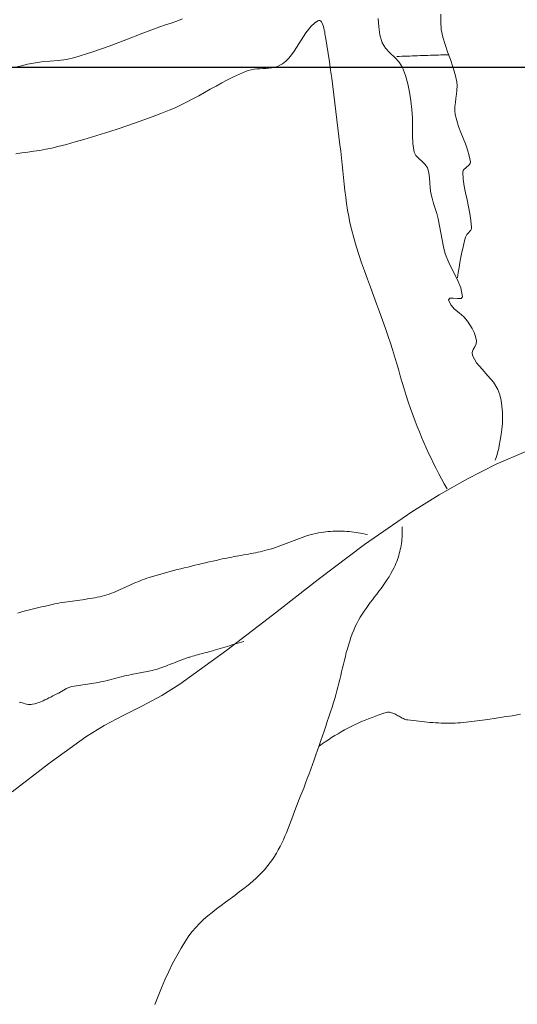
# Model space of a CAD drawing. Units: inches. Extents: x 1484 to 2008, y 1843 to 2590.
# Tile 15 of 21: x 1817 to 1832, y 2172 to 2201. Entities that reach past the tile are written whole.
import ezdxf

# ---------------------------------------------------------------- set-up
doc = ezdxf.new("R2010")
doc.units = ezdxf.units.IN
doc.layers.add('A-ANNO-DIMS', color=2, linetype='Continuous', lineweight=18)
doc.layers.add('A-FURN', color=8, linetype='Continuous', lineweight=18)
doc.styles.get("Standard").update_dxf_attribs({"font": 'arial.ttf'})
doc.dimstyles.new('ISO-25', dxfattribs={"dimtxt": 7, "dimasz": 2.5, "dimexe": 1.25, "dimexo": 0.625, "dimtad": 1, "dimdec": 0, "dimlunit": 3, "dimtxsty": 'Standard', "dimcen": 2.5, "dimadec": 0, "dimazin": 0, "dimtfac": 1, "dimtdec": 0, "dimtmove": 0, "dimatfit": 3, "dimfxl": 1, "dimarcsym": 0})

# ---------------------------------------------------------------- blocks, each defined once
blk = doc.blocks.new('BED-DOUBLE')
for p, q in [((27.086, 81.663), (27.081, 81.437)), ((18.331, 81.099), (18.829, 81.285)), ((18.829, 81.285), (18.997, 81.343)), ((18.997, 81.343), (19.165, 81.4)), ((19.165, 81.4), (19.333, 81.457)), ((19.333, 81.457), (19.499, 81.518)), ((23.197, 81.214), (23.28, 81.307)), ((23.28, 81.307), (23.371, 81.391)), ((23.371, 81.391), (23.472, 81.464)), ((23.472, 81.464), (23.504, 81.477)), ((23.504, 81.477), (23.533, 81.475)), ((23.533, 81.475), (23.559, 81.459)), ((23.559, 81.459), (23.582, 81.432)), ((23.582, 81.432), (23.603, 81.395)), ((23.603, 81.395), (23.621, 81.351)), ((23.621, 81.351), (23.637, 81.301)), ((23.637, 81.301), (23.65, 81.248)), ((25.241, 81.536), (25.262, 81.291)), ((25.262, 81.291), (25.297, 81.049)), ((27.081, 81.437), (27.1, 81.21)), ((17.835, 80.908), (18.331, 81.099)), ((22.98, 80.898), (23.048, 81.007)), ((23.048, 81.007), (23.12, 81.113)), ((23.12, 81.113), (23.197, 81.214)), ((23.65, 81.248), (23.662, 81.193)), ((23.662, 81.193), (23.673, 81.137)), ((23.673, 81.137), (23.682, 81.084)), ((23.682, 81.084), (23.69, 81.035)), ((23.69, 81.035), (23.698, 80.992)), ((23.698, 80.992), (23.739, 80.749)), ((25.297, 81.049), (25.366, 80.818)), ((27.1, 81.21), (27.146, 80.988)), ((27.146, 80.988), (27.21, 80.768)), ((16.837, 80.542), (17.338, 80.72)), ((17.338, 80.72), (17.835, 80.908)), ((22.844, 80.677), (22.912, 80.787)), ((22.912, 80.787), (22.98, 80.898)), ((23.739, 80.749), (23.778, 80.506)), ((25.366, 80.818), (25.462, 80.659)), ((27.21, 80.768), (27.285, 80.55)), ((16.33, 80.384), (16.837, 80.542)), ((22.618, 80.369), (22.698, 80.466)), ((22.698, 80.466), (22.773, 80.569)), ((22.773, 80.569), (22.844, 80.677)), ((23.778, 80.506), (23.814, 80.263)), ((25.462, 80.659), (25.591, 80.52)), ((25.591, 80.52), (25.731, 80.387)), ((25.788, 80.416), (25.865, 80.419)), ((25.865, 80.419), (25.941, 80.422)), ((25.941, 80.422), (26.018, 80.424)), ((26.018, 80.424), (26.094, 80.427)), ((26.094, 80.427), (26.171, 80.43)), ((26.171, 80.43), (26.247, 80.433)), ((26.247, 80.433), (26.324, 80.435)), ((26.324, 80.435), (26.401, 80.438)), ((26.401, 80.438), (26.477, 80.441)), ((26.477, 80.441), (26.554, 80.443)), ((26.554, 80.443), (26.63, 80.446)), ((26.63, 80.446), (26.707, 80.449)), ((26.707, 80.449), (26.783, 80.451)), ((26.783, 80.451), (26.86, 80.454)), ((26.86, 80.454), (26.936, 80.457)), ((26.936, 80.457), (27.013, 80.459)), ((27.013, 80.459), (27.09, 80.462)), ((27.09, 80.462), (27.166, 80.465)), ((27.166, 80.465), (27.243, 80.468)), ((27.243, 80.468), (27.319, 80.47)), ((27.285, 80.55), (27.365, 80.332)), ((14.594, 80.099), (14.766, 80.146)), ((14.766, 80.146), (14.94, 80.187)), ((14.94, 80.187), (15.115, 80.222)), ((15.115, 80.222), (15.357, 80.259)), ((15.357, 80.259), (15.602, 80.281)), ((15.602, 80.281), (15.848, 80.302)), ((15.848, 80.302), (16.091, 80.332)), ((16.091, 80.332), (16.33, 80.384)), ((22.204, 80.103), (22.283, 80.127)), ((22.283, 80.127), (22.36, 80.16)), ((22.36, 80.16), (22.432, 80.203)), ((22.432, 80.203), (22.529, 80.281)), ((22.529, 80.281), (22.618, 80.369)), ((23.814, 80.263), (23.848, 80.019)), ((25.731, 80.387), (25.862, 80.249)), ((25.862, 80.249), (25.961, 80.091)), ((27.365, 80.332), (27.441, 80.113)), ((20.996, 79.819), (21.172, 79.902)), ((21.172, 79.902), (21.349, 79.979)), ((21.349, 79.979), (21.43, 80.007)), ((21.43, 80.007), (21.513, 80.027)), ((21.513, 80.027), (21.598, 80.04)), ((21.598, 80.04), (21.685, 80.05)), ((21.685, 80.05), (21.773, 80.056)), ((21.773, 80.056), (21.861, 80.061)), ((21.861, 80.061), (21.949, 80.067)), ((21.949, 80.067), (22.036, 80.075)), ((22.036, 80.075), (22.121, 80.086)), ((22.121, 80.086), (22.204, 80.103)), ((23.848, 80.019), (23.88, 79.776)), ((25.961, 80.091), (26.05, 79.856)), ((26.05, 79.856), (26.116, 79.613)), ((27.441, 80.113), (27.506, 79.892)), ((27.506, 79.892), (27.553, 79.668)), ((20.312, 79.453), (20.482, 79.548)), ((20.482, 79.548), (20.652, 79.641)), ((20.652, 79.641), (20.823, 79.732)), ((20.823, 79.732), (20.996, 79.819)), ((23.88, 79.776), (23.911, 79.531)), ((26.116, 79.613), (26.165, 79.364)), ((27.553, 79.668), (27.563, 79.55)), ((27.563, 79.55), (27.56, 79.43)), ((19.802, 79.17), (19.973, 79.263)), ((19.973, 79.263), (20.143, 79.358)), ((20.143, 79.358), (20.312, 79.453)), ((23.911, 79.531), (23.941, 79.287)), ((23.941, 79.287), (23.97, 79.043)), ((26.165, 79.364), (26.203, 79.113)), ((27.547, 79.31), (27.53, 79.19)), ((27.56, 79.43), (27.547, 79.31)), ((19.282, 78.912), (19.457, 78.993)), ((19.457, 78.993), (19.631, 79.08)), ((19.631, 79.08), (19.802, 79.17)), ((23.97, 79.043), (23.999, 78.798)), ((26.203, 79.113), (26.238, 78.862)), ((27.513, 79.069), (27.501, 78.95)), ((27.53, 79.19), (27.513, 79.069)), ((18.61, 78.645), (18.857, 78.739)), ((18.857, 78.739), (19.103, 78.836)), ((19.103, 78.836), (19.282, 78.912)), ((23.999, 78.798), (24.028, 78.554)), ((26.238, 78.862), (26.256, 78.612)), ((27.501, 78.95), (27.499, 78.83)), ((27.499, 78.83), (27.51, 78.712)), ((27.51, 78.712), (27.551, 78.534)), ((17.862, 78.377), (18.112, 78.464)), ((18.112, 78.464), (18.362, 78.553)), ((18.362, 78.553), (18.61, 78.645)), ((24.028, 78.554), (24.058, 78.31)), ((26.256, 78.612), (26.254, 78.359)), ((27.551, 78.534), (27.606, 78.36)), ((16.853, 78.054), (17.107, 78.131)), ((17.107, 78.131), (17.359, 78.21)), ((17.359, 78.21), (17.611, 78.292)), ((17.611, 78.292), (17.862, 78.377)), ((24.058, 78.31), (24.089, 78.066)), ((26.254, 78.359), (26.249, 78.107)), ((26.249, 78.107), (26.259, 77.856)), ((27.606, 78.36), (27.671, 78.188)), ((27.671, 78.188), (27.74, 78.018)), ((15.833, 77.768), (16.089, 77.836)), ((16.089, 77.836), (16.344, 77.906)), ((16.344, 77.906), (16.599, 77.979)), ((16.599, 77.979), (16.853, 78.054)), ((24.089, 78.066), (24.121, 77.822)), ((24.121, 77.822), (24.145, 77.631)), ((26.259, 77.856), (26.301, 77.611)), ((27.74, 78.018), (27.809, 77.847)), ((27.809, 77.847), (27.871, 77.675)), ((14.596, 77.562), (14.774, 77.584)), ((14.774, 77.584), (14.953, 77.607)), ((14.953, 77.607), (15.13, 77.632)), ((15.13, 77.632), (15.308, 77.659)), ((15.308, 77.659), (15.484, 77.69)), ((15.484, 77.69), (15.659, 77.726)), ((15.659, 77.726), (15.833, 77.768)), ((24.145, 77.631), (24.167, 77.439)), ((26.301, 77.611), (26.354, 77.505)), ((27.871, 77.675), (27.922, 77.5)), ((24.167, 77.439), (24.188, 77.247)), ((24.188, 77.247), (24.207, 77.055)), ((26.354, 77.505), (26.439, 77.416)), ((26.439, 77.416), (26.536, 77.332)), ((26.536, 77.332), (26.627, 77.245)), ((26.627, 77.245), (26.692, 77.143)), ((27.928, 77.24), (27.892, 77.205)), ((27.922, 77.5), (27.956, 77.322)), ((27.951, 77.278), (27.928, 77.24)), ((27.956, 77.322), (27.951, 77.278)), ((24.207, 77.055), (24.226, 76.863)), ((26.692, 77.143), (26.733, 77.001)), ((26.733, 77.001), (26.753, 76.853)), ((27.743, 77.064), (27.733, 77.02)), ((27.733, 77.02), (27.745, 76.815)), ((27.769, 77.102), (27.743, 77.064)), ((27.807, 77.138), (27.769, 77.102)), ((27.85, 77.171), (27.807, 77.138)), ((27.892, 77.205), (27.85, 77.171)), ((24.226, 76.863), (24.246, 76.671)), ((24.246, 76.671), (24.267, 76.479)), ((26.753, 76.853), (26.761, 76.702)), ((26.761, 76.702), (26.771, 76.552)), ((27.745, 76.815), (27.773, 76.611)), ((24.267, 76.479), (24.29, 76.288)), ((26.771, 76.552), (26.792, 76.404)), ((26.792, 76.404), (26.83, 76.252)), ((27.773, 76.611), (27.811, 76.409)), ((27.811, 76.409), (27.854, 76.207)), ((24.29, 76.288), (24.316, 76.097)), ((24.316, 76.097), (24.346, 75.907)), ((26.83, 76.252), (26.874, 76.101)), ((26.874, 76.101), (26.922, 75.952)), ((27.854, 76.207), (27.899, 76.005)), ((24.346, 75.907), (24.379, 75.717)), ((26.922, 75.952), (26.968, 75.802)), ((26.968, 75.802), (27.008, 75.651)), ((27.899, 76.005), (27.939, 75.803)), ((27.939, 75.803), (27.97, 75.599)), ((24.379, 75.717), (24.417, 75.529)), ((24.417, 75.529), (24.461, 75.342)), ((27.008, 75.651), (27.051, 75.444)), ((27.97, 75.599), (27.987, 75.395)), ((24.461, 75.342), (24.527, 75.094)), ((27.051, 75.444), (27.086, 75.236)), ((27.086, 75.236), (27.12, 75.028)), ((27.882, 75.218), (27.853, 75.184)), ((27.912, 75.251), (27.882, 75.218)), ((27.941, 75.284), (27.912, 75.251)), ((27.966, 75.318), (27.941, 75.284)), ((27.982, 75.355), (27.966, 75.318)), ((27.987, 75.395), (27.982, 75.355)), ((24.527, 75.094), (24.599, 74.848)), ((27.12, 75.028), (27.161, 74.821)), ((27.773, 74.963), (27.737, 74.816)), ((27.812, 75.11), (27.773, 74.963)), ((27.829, 75.149), (27.812, 75.11)), ((27.853, 75.184), (27.829, 75.149)), ((24.599, 74.848), (24.676, 74.603)), ((27.161, 74.821), (27.215, 74.618)), ((27.703, 74.667), (27.672, 74.518)), ((27.737, 74.816), (27.703, 74.667)), ((24.676, 74.603), (24.757, 74.36)), ((24.757, 74.36), (24.842, 74.118)), ((27.215, 74.618), (27.316, 74.365)), ((27.316, 74.365), (27.442, 74.119)), ((27.644, 74.369), (27.619, 74.219)), ((27.672, 74.518), (27.644, 74.369)), ((24.842, 74.118), (24.929, 73.877)), ((27.442, 74.119), (27.569, 73.874)), ((27.597, 74.069), (27.578, 73.918)), ((27.619, 74.219), (27.597, 74.069)), ((24.929, 73.877), (25.018, 73.636)), ((27.569, 73.874), (27.67, 73.623)), ((25.018, 73.636), (25.108, 73.395)), ((27.67, 73.623), (27.723, 73.361)), ((25.108, 73.395), (25.198, 73.155)), ((27.346, 73.318), (27.313, 73.269)), ((27.313, 73.269), (27.378, 73.12)), ((27.448, 73.32), (27.346, 73.318)), ((27.575, 73.308), (27.448, 73.32)), ((27.682, 73.311), (27.575, 73.308)), ((27.723, 73.361), (27.682, 73.311)), ((25.198, 73.155), (25.288, 72.914)), ((25.288, 72.914), (25.375, 72.673)), ((27.378, 73.12), (27.489, 72.995)), ((27.489, 72.995), (27.624, 72.882)), ((25.375, 72.673), (25.461, 72.431)), ((27.624, 72.882), (27.759, 72.768)), ((27.759, 72.768), (27.872, 72.64)), ((27.872, 72.64), (27.942, 72.534)), ((25.461, 72.431), (25.543, 72.188)), ((27.942, 72.534), (28.007, 72.424)), ((28.007, 72.424), (28.063, 72.31)), ((28.063, 72.31), (28.107, 72.192)), ((25.543, 72.188), (25.605, 71.997)), ((28.107, 72.192), (28.134, 72.069)), ((28.134, 72.069), (28.123, 71.981)), ((25.605, 71.997), (25.665, 71.805)), ((25.665, 71.805), (25.723, 71.613)), ((28.035, 71.806), (28.004, 71.721)), ((28.082, 71.893), (28.035, 71.806)), ((28.123, 71.981), (28.082, 71.893)), ((25.723, 71.613), (25.78, 71.421)), ((28.004, 71.721), (28.012, 71.638)), ((28.012, 71.638), (28.137, 71.423)), ((25.78, 71.421), (25.837, 71.228)), ((25.837, 71.228), (25.893, 71.036)), ((28.137, 71.423), (28.296, 71.228)), ((28.296, 71.228), (28.468, 71.04)), ((25.893, 71.036), (25.95, 70.843)), ((28.468, 71.04), (28.63, 70.847)), ((25.95, 70.843), (26.008, 70.651)), ((26.008, 70.651), (26.067, 70.46)), ((28.63, 70.847), (28.762, 70.635)), ((28.762, 70.635), (28.822, 70.477)), ((26.067, 70.46), (26.128, 70.269)), ((28.822, 70.477), (28.86, 70.311)), ((28.86, 70.311), (28.882, 70.141)), ((26.128, 70.269), (26.192, 70.079)), ((26.192, 70.079), (26.259, 69.89)), ((28.882, 70.141), (28.892, 69.969)), ((26.259, 69.89), (26.329, 69.702)), ((28.892, 69.969), (28.897, 69.797)), ((28.897, 69.797), (28.894, 69.635)), ((26.329, 69.702), (26.391, 69.545)), ((26.391, 69.545), (26.454, 69.388)), ((28.88, 69.472), (28.858, 69.31)), ((28.894, 69.635), (28.88, 69.472)), ((26.454, 69.388), (26.52, 69.232)), ((26.52, 69.232), (26.587, 69.076)), ((28.83, 69.149), (28.802, 68.988)), ((28.858, 69.31), (28.83, 69.149)), ((26.587, 69.076), (26.655, 68.922)), ((26.655, 68.922), (26.726, 68.768)), ((28.785, 68.9), (28.764, 68.812)), ((28.802, 68.988), (28.785, 68.9)), ((26.726, 68.768), (26.798, 68.615)), ((26.798, 68.615), (26.872, 68.462)), ((28.712, 68.64), (28.68, 68.556)), ((29.579, 68.813), (28.71, 68.44)), ((28.739, 68.726), (28.712, 68.64)), ((28.764, 68.812), (28.739, 68.726)), ((26.872, 68.462), (26.948, 68.311)), ((26.948, 68.311), (27.025, 68.16)), ((28.71, 68.44), (27.864, 68.011)), ((27.025, 68.16), (27.104, 68.011)), ((27.864, 68.011), (27.04, 67.54)), ((27.104, 68.011), (27.185, 67.862)), ((27.185, 67.862), (27.267, 67.714)), ((27.04, 67.54), (26.237, 67.038)), ((26.237, 67.038), (24.84, 66.077)), ((25.954, 66.542), (25.951, 66.603)), ((25.954, 66.481), (25.954, 66.542)), ((22.855, 66.232), (22.777, 66.202)), ((22.933, 66.261), (22.855, 66.232)), ((23.012, 66.289), (22.933, 66.261)), ((23.091, 66.316), (23.012, 66.289)), ((23.17, 66.342), (23.091, 66.316)), ((23.25, 66.366), (23.17, 66.342)), ((23.33, 66.387), (23.25, 66.366)), ((23.411, 66.407), (23.33, 66.387)), ((23.492, 66.424), (23.411, 66.407)), ((23.574, 66.438), (23.492, 66.424)), ((23.641, 66.448), (23.574, 66.438)), ((23.709, 66.456), (23.641, 66.448)), ((23.776, 66.463), (23.709, 66.456)), ((23.844, 66.468), (23.776, 66.463)), ((23.912, 66.472), (23.844, 66.468)), ((23.981, 66.475), (23.912, 66.472)), ((24.049, 66.476), (23.981, 66.475)), ((24.117, 66.476), (24.049, 66.476)), ((24.186, 66.475), (24.117, 66.476)), ((24.254, 66.472), (24.186, 66.475)), ((24.322, 66.468), (24.254, 66.472)), ((24.39, 66.463), (24.322, 66.468)), ((24.458, 66.456), (24.39, 66.463)), ((24.526, 66.448), (24.458, 66.456)), ((24.594, 66.439), (24.526, 66.448)), ((24.661, 66.428), (24.594, 66.439)), ((24.728, 66.416), (24.661, 66.428)), ((24.795, 66.403), (24.728, 66.416)), ((24.861, 66.388), (24.795, 66.403)), ((24.927, 66.372), (24.861, 66.388)), ((25.935, 66.175), (25.942, 66.236)), ((25.942, 66.236), (25.948, 66.298)), ((25.948, 66.298), (25.951, 66.359)), ((25.951, 66.359), (25.954, 66.42)), ((25.954, 66.42), (25.954, 66.481)), ((22.069, 65.944), (21.988, 65.921)), ((22.148, 65.969), (22.069, 65.944)), ((22.228, 65.995), (22.148, 65.969)), ((22.307, 66.022), (22.228, 65.995)), ((22.385, 66.051), (22.307, 66.022)), ((22.464, 66.081), (22.385, 66.051)), ((22.542, 66.111), (22.464, 66.081)), ((22.62, 66.141), (22.542, 66.111)), ((22.698, 66.172), (22.62, 66.141)), ((22.777, 66.202), (22.698, 66.172)), ((24.84, 66.077), (23.483, 65.057)), ((25.894, 65.932), (25.906, 65.993)), ((25.906, 65.993), (25.917, 66.053)), ((25.917, 66.053), (25.927, 66.114)), ((25.927, 66.114), (25.935, 66.175)), ((20.664, 65.656), (20.594, 65.64)), ((20.733, 65.671), (20.664, 65.656)), ((20.803, 65.685), (20.733, 65.671)), ((20.873, 65.699), (20.803, 65.685)), ((20.943, 65.712), (20.873, 65.699)), ((21.013, 65.725), (20.943, 65.712)), ((21.083, 65.738), (21.013, 65.725)), ((21.153, 65.751), (21.083, 65.738)), ((21.223, 65.763), (21.153, 65.751)), ((21.293, 65.775), (21.223, 65.763)), ((21.363, 65.788), (21.293, 65.775)), ((21.433, 65.801), (21.363, 65.788)), ((21.503, 65.814), (21.433, 65.801)), ((21.573, 65.827), (21.503, 65.814)), ((21.642, 65.841), (21.573, 65.827)), ((21.712, 65.856), (21.642, 65.841)), ((21.781, 65.871), (21.712, 65.856)), ((21.851, 65.887), (21.781, 65.871)), ((21.92, 65.904), (21.851, 65.887)), ((21.988, 65.921), (21.92, 65.904)), ((25.809, 65.637), (25.829, 65.695)), ((25.829, 65.695), (25.847, 65.754)), ((25.847, 65.754), (25.864, 65.813)), ((25.864, 65.813), (25.88, 65.872)), ((25.88, 65.872), (25.894, 65.932)), ((19.445, 65.369), (19.341, 65.343)), ((19.549, 65.395), (19.445, 65.369)), ((19.654, 65.42), (19.549, 65.395)), ((19.758, 65.445), (19.654, 65.42)), ((19.863, 65.47), (19.758, 65.445)), ((19.967, 65.495), (19.863, 65.47)), ((20.072, 65.519), (19.967, 65.495)), ((20.176, 65.543), (20.072, 65.519)), ((20.281, 65.568), (20.176, 65.543)), ((20.385, 65.592), (20.281, 65.568)), ((20.49, 65.616), (20.385, 65.592)), ((20.594, 65.64), (20.49, 65.616)), ((25.67, 65.318), (25.717, 65.411)), ((25.717, 65.411), (25.742, 65.466)), ((25.742, 65.466), (25.766, 65.522)), ((25.766, 65.522), (25.788, 65.579)), ((25.788, 65.579), (25.809, 65.637)), ((18.448, 65.09), (18.381, 65.067)), ((18.515, 65.112), (18.448, 65.09)), ((18.617, 65.143), (18.515, 65.112)), ((18.72, 65.174), (18.617, 65.143)), ((18.823, 65.204), (18.72, 65.174)), ((18.926, 65.233), (18.823, 65.204)), ((19.03, 65.261), (18.926, 65.233)), ((19.133, 65.289), (19.03, 65.261)), ((19.237, 65.316), (19.133, 65.289)), ((19.341, 65.343), (19.237, 65.316)), ((25.512, 65.049), (25.568, 65.137)), ((25.568, 65.137), (25.621, 65.226)), ((25.621, 65.226), (25.67, 65.318)), ((17.735, 64.785), (17.67, 64.757)), ((17.799, 64.815), (17.735, 64.785)), ((17.863, 64.844), (17.799, 64.815)), ((17.927, 64.873), (17.863, 64.844)), ((17.992, 64.903), (17.927, 64.873)), ((18.056, 64.932), (17.992, 64.903)), ((18.12, 64.961), (18.056, 64.932)), ((18.185, 64.989), (18.12, 64.961)), ((18.25, 65.016), (18.185, 64.989)), ((18.316, 65.042), (18.25, 65.016)), ((18.381, 65.067), (18.316, 65.042)), ((23.483, 65.057), (22.143, 64.011)), ((25.268, 64.709), (25.331, 64.793)), ((25.331, 64.793), (25.393, 64.877)), ((25.393, 64.877), (25.453, 64.963)), ((25.453, 64.963), (25.512, 65.049)), ((16.848, 64.505), (16.775, 64.492)), ((16.921, 64.518), (16.848, 64.505)), ((16.993, 64.533), (16.921, 64.518)), ((17.066, 64.549), (16.993, 64.533)), ((17.138, 64.567), (17.066, 64.549)), ((17.209, 64.586), (17.138, 64.567)), ((17.277, 64.606), (17.209, 64.586)), ((17.343, 64.627), (17.277, 64.606)), ((17.41, 64.651), (17.343, 64.627)), ((17.475, 64.676), (17.41, 64.651)), ((17.541, 64.702), (17.475, 64.676)), ((17.606, 64.729), (17.541, 64.702)), ((17.67, 64.757), (17.606, 64.729)), ((25.077, 64.458), (25.141, 64.542)), ((25.141, 64.542), (25.205, 64.625)), ((25.205, 64.625), (25.268, 64.709)), ((15.195, 64.209), (15.116, 64.189)), ((15.274, 64.228), (15.195, 64.209)), ((15.353, 64.247), (15.274, 64.228)), ((15.432, 64.265), (15.353, 64.247)), ((15.511, 64.283), (15.432, 64.265)), ((15.59, 64.301), (15.511, 64.283)), ((15.669, 64.319), (15.59, 64.301)), ((15.749, 64.336), (15.669, 64.319)), ((15.821, 64.351), (15.749, 64.336)), ((15.894, 64.364), (15.821, 64.351)), ((15.967, 64.377), (15.894, 64.364)), ((16.04, 64.389), (15.967, 64.377)), ((16.114, 64.4), (16.04, 64.389)), ((16.187, 64.41), (16.114, 64.4)), ((16.261, 64.42), (16.187, 64.41)), ((16.334, 64.43), (16.261, 64.42)), ((16.408, 64.44), (16.334, 64.43)), ((16.482, 64.45), (16.408, 64.44)), ((16.555, 64.46), (16.482, 64.45)), ((16.629, 64.47), (16.555, 64.46)), ((16.702, 64.481), (16.629, 64.47)), ((16.775, 64.492), (16.702, 64.481)), ((24.89, 64.206), (24.951, 64.291)), ((24.951, 64.291), (25.013, 64.375)), ((25.013, 64.375), (25.077, 64.458)), ((14.723, 64.088), (14.645, 64.067)), ((14.802, 64.109), (14.723, 64.088)), ((14.88, 64.129), (14.802, 64.109)), ((14.959, 64.15), (14.88, 64.129)), ((15.038, 64.17), (14.959, 64.15)), ((15.116, 64.189), (15.038, 64.17)), ((22.143, 64.011), (20.798, 62.974)), ((24.666, 63.855), (24.718, 63.945)), ((24.718, 63.945), (24.773, 64.033)), ((24.773, 64.033), (24.83, 64.12)), ((24.83, 64.12), (24.89, 64.206)), ((24.527, 63.563), (24.573, 63.669)), ((24.573, 63.669), (24.617, 63.763)), ((24.617, 63.763), (24.666, 63.855)), ((24.408, 63.238), (24.445, 63.347)), ((24.445, 63.347), (24.484, 63.456)), ((24.484, 63.456), (24.527, 63.563)), ((20.743, 63.068), (20.673, 63.047)), ((20.812, 63.088), (20.743, 63.068)), ((20.881, 63.109), (20.812, 63.088)), ((20.95, 63.13), (20.881, 63.109)), ((21.019, 63.151), (20.95, 63.13)), ((21.088, 63.172), (21.019, 63.151)), ((21.158, 63.193), (21.088, 63.172)), ((21.227, 63.214), (21.158, 63.193)), ((21.296, 63.235), (21.227, 63.214)), ((24.34, 63.017), (24.373, 63.128)), ((24.373, 63.128), (24.408, 63.238)), ((20.798, 62.974), (19.423, 61.978)), ((19.688, 62.768), (19.661, 62.759)), ((19.714, 62.777), (19.688, 62.768)), ((19.741, 62.785), (19.714, 62.777)), ((19.791, 62.8), (19.741, 62.785)), ((19.841, 62.815), (19.791, 62.8)), ((19.892, 62.829), (19.841, 62.815)), ((19.942, 62.843), (19.892, 62.829)), ((19.992, 62.857), (19.942, 62.843)), ((20.043, 62.87), (19.992, 62.857)), ((20.093, 62.883), (20.043, 62.87)), ((20.144, 62.897), (20.093, 62.883)), ((20.194, 62.91), (20.144, 62.897)), ((20.245, 62.924), (20.194, 62.91)), ((20.295, 62.938), (20.245, 62.924)), ((20.346, 62.952), (20.295, 62.938)), ((20.396, 62.966), (20.346, 62.952)), ((20.465, 62.986), (20.396, 62.966)), ((20.535, 63.006), (20.465, 62.986)), ((20.604, 63.027), (20.535, 63.006)), ((20.673, 63.047), (20.604, 63.027)), ((24.252, 62.681), (24.28, 62.794)), ((24.28, 62.794), (24.309, 62.906)), ((24.309, 62.906), (24.34, 63.017)), ((18.948, 62.491), (18.892, 62.47)), ((19.005, 62.512), (18.948, 62.491)), ((19.061, 62.533), (19.005, 62.512)), ((19.117, 62.555), (19.061, 62.533)), ((19.173, 62.577), (19.117, 62.555)), ((19.229, 62.598), (19.173, 62.577)), ((19.285, 62.62), (19.229, 62.598)), ((19.342, 62.641), (19.285, 62.62)), ((19.398, 62.662), (19.342, 62.641)), ((19.425, 62.671), (19.398, 62.662)), ((19.451, 62.681), (19.425, 62.671)), ((19.477, 62.691), (19.451, 62.681)), ((19.503, 62.701), (19.477, 62.691)), ((19.53, 62.711), (19.503, 62.701)), ((19.556, 62.721), (19.53, 62.711)), ((19.582, 62.73), (19.556, 62.721)), ((19.608, 62.74), (19.582, 62.73)), ((19.635, 62.75), (19.608, 62.74)), ((19.661, 62.759), (19.635, 62.75)), ((24.197, 62.456), (24.224, 62.569)), ((24.224, 62.569), (24.252, 62.681)), ((17.693, 62.192), (17.619, 62.173)), ((17.767, 62.211), (17.693, 62.192)), ((17.842, 62.23), (17.767, 62.211)), ((17.916, 62.247), (17.842, 62.23)), ((17.991, 62.265), (17.916, 62.247)), ((18.042, 62.276), (17.991, 62.265)), ((18.094, 62.286), (18.042, 62.276)), ((18.146, 62.296), (18.094, 62.286)), ((18.198, 62.305), (18.146, 62.296)), ((18.25, 62.313), (18.198, 62.305)), ((18.302, 62.322), (18.25, 62.313)), ((18.354, 62.331), (18.302, 62.322)), ((18.406, 62.34), (18.354, 62.331)), ((18.458, 62.349), (18.406, 62.34)), ((18.509, 62.359), (18.458, 62.349)), ((18.561, 62.371), (18.509, 62.359)), ((18.612, 62.383), (18.561, 62.371)), ((18.663, 62.396), (18.612, 62.383)), ((18.721, 62.413), (18.663, 62.396)), ((18.778, 62.431), (18.721, 62.413)), ((18.835, 62.45), (18.778, 62.431)), ((18.892, 62.47), (18.835, 62.45)), ((24.118, 62.116), (24.144, 62.229)), ((24.144, 62.229), (24.171, 62.343)), ((24.171, 62.343), (24.197, 62.456)), ((16.25, 61.907), (16.187, 61.891)), ((16.314, 61.92), (16.25, 61.907)), ((16.378, 61.932), (16.314, 61.92)), ((16.443, 61.943), (16.378, 61.932)), ((16.507, 61.952), (16.443, 61.943)), ((16.572, 61.961), (16.507, 61.952)), ((16.637, 61.969), (16.572, 61.961)), ((16.702, 61.977), (16.637, 61.969)), ((16.766, 61.985), (16.702, 61.977)), ((16.831, 61.994), (16.766, 61.985)), ((16.896, 62.004), (16.831, 61.994)), ((16.96, 62.015), (16.896, 62.004)), ((17.024, 62.027), (16.96, 62.015)), ((17.099, 62.043), (17.024, 62.027)), ((17.174, 62.06), (17.099, 62.043)), ((17.248, 62.078), (17.174, 62.06)), ((17.322, 62.096), (17.248, 62.078)), ((17.397, 62.115), (17.322, 62.096)), ((17.471, 62.134), (17.397, 62.115)), ((17.545, 62.153), (17.471, 62.134)), ((17.619, 62.173), (17.545, 62.153)), ((19.423, 61.978), (18.885, 61.644)), ((24.062, 61.891), (24.09, 62.004)), ((24.09, 62.004), (24.118, 62.116)), ((15.688, 61.632), (15.631, 61.602)), ((15.746, 61.662), (15.688, 61.632)), ((15.804, 61.691), (15.746, 61.662)), ((15.862, 61.719), (15.804, 61.691)), ((15.887, 61.731), (15.862, 61.719)), ((15.912, 61.745), (15.887, 61.731)), ((15.937, 61.759), (15.912, 61.745)), ((15.961, 61.774), (15.937, 61.759)), ((15.985, 61.789), (15.961, 61.774)), ((16.01, 61.805), (15.985, 61.789)), ((16.034, 61.82), (16.01, 61.805)), ((16.058, 61.835), (16.034, 61.82)), ((16.083, 61.848), (16.058, 61.835)), ((16.108, 61.861), (16.083, 61.848)), ((16.134, 61.873), (16.108, 61.861)), ((16.16, 61.883), (16.134, 61.873)), ((16.187, 61.891), (16.16, 61.883)), ((18.885, 61.644), (18.326, 61.345)), ((23.969, 61.556), (24.002, 61.667)), ((24.002, 61.667), (24.033, 61.779)), ((24.033, 61.779), (24.062, 61.891)), ((14.738, 61.442), (14.694, 61.452)), ((14.783, 61.43), (14.738, 61.442)), ((14.828, 61.418), (14.783, 61.43)), ((14.873, 61.405), (14.828, 61.418)), ((14.918, 61.395), (14.873, 61.405)), ((14.962, 61.386), (14.918, 61.395)), ((15.007, 61.382), (14.962, 61.386)), ((15.051, 61.381), (15.007, 61.382)), ((15.095, 61.387), (15.051, 61.381)), ((15.158, 61.401), (15.095, 61.387)), ((15.219, 61.419), (15.158, 61.401)), ((15.28, 61.439), (15.219, 61.419)), ((15.339, 61.462), (15.28, 61.439)), ((15.399, 61.488), (15.339, 61.462)), ((15.457, 61.515), (15.399, 61.488)), ((15.515, 61.543), (15.457, 61.515)), ((15.573, 61.573), (15.515, 61.543)), ((15.631, 61.602), (15.573, 61.573)), ((18.326, 61.345), (17.758, 61.059)), ((23.889, 61.305), (23.935, 61.445)), ((23.935, 61.445), (23.969, 61.556)), ((17.758, 61.059), (17.198, 60.761)), ((23.797, 61.023), (23.843, 61.164)), ((23.843, 61.164), (23.889, 61.305)), ((25.168, 61.043), (25.064, 61.005)), ((25.272, 61.079), (25.168, 61.043)), ((25.377, 61.113), (25.272, 61.079)), ((25.483, 61.145), (25.377, 61.113)), ((25.515, 61.153), (25.483, 61.145)), ((25.546, 61.155), (25.515, 61.153)), ((25.578, 61.154), (25.546, 61.155)), ((25.609, 61.15), (25.578, 61.154)), ((25.64, 61.142), (25.609, 61.15)), ((25.671, 61.132), (25.64, 61.142)), ((25.703, 61.12), (25.671, 61.132)), ((25.734, 61.105), (25.703, 61.12)), ((25.765, 61.089), (25.734, 61.105)), ((25.796, 61.072), (25.765, 61.089)), ((25.827, 61.054), (25.796, 61.072)), ((25.858, 61.036), (25.827, 61.054)), ((25.889, 61.018), (25.858, 61.036)), ((29.183, 61.054), (28.945, 61.015)), ((29.421, 61.095), (29.183, 61.054)), ((17.198, 60.761), (16.659, 60.428)), ((23.657, 60.601), (23.704, 60.742)), ((23.704, 60.742), (23.751, 60.882)), ((23.751, 60.882), (23.797, 61.023)), ((24.455, 60.738), (24.356, 60.687)), ((24.554, 60.787), (24.455, 60.738)), ((24.655, 60.834), (24.554, 60.787)), ((24.756, 60.879), (24.655, 60.834)), ((24.858, 60.923), (24.756, 60.879)), ((24.961, 60.965), (24.858, 60.923)), ((25.064, 61.005), (24.961, 60.965)), ((25.921, 61.001), (25.889, 61.018)), ((25.952, 60.985), (25.921, 61.001)), ((25.984, 60.969), (25.952, 60.985)), ((26.016, 60.956), (25.984, 60.969)), ((26.049, 60.945), (26.016, 60.956)), ((26.081, 60.936), (26.049, 60.945)), ((26.114, 60.93), (26.081, 60.936)), ((26.195, 60.92), (26.114, 60.93)), ((26.277, 60.91), (26.195, 60.92)), ((26.358, 60.9), (26.277, 60.91)), ((26.44, 60.89), (26.358, 60.9)), ((26.521, 60.881), (26.44, 60.89)), ((26.603, 60.873), (26.521, 60.881)), ((26.685, 60.865), (26.603, 60.873)), ((26.766, 60.858), (26.685, 60.865)), ((26.848, 60.851), (26.766, 60.858)), ((26.93, 60.846), (26.848, 60.851)), ((27.012, 60.841), (26.93, 60.846)), ((27.094, 60.837), (27.012, 60.841)), ((27.176, 60.835), (27.094, 60.837)), ((27.258, 60.833), (27.176, 60.835)), ((27.339, 60.833), (27.258, 60.833)), ((27.421, 60.834), (27.339, 60.833)), ((27.503, 60.837), (27.421, 60.834)), ((27.585, 60.841), (27.503, 60.837)), ((27.666, 60.847), (27.585, 60.841)), ((27.747, 60.854), (27.666, 60.847)), ((27.988, 60.881), (27.747, 60.854)), ((28.227, 60.91), (27.988, 60.881)), ((28.467, 60.943), (28.227, 60.91)), ((28.706, 60.978), (28.467, 60.943)), ((28.945, 61.015), (28.706, 60.978)), ((23.562, 60.321), (23.61, 60.461)), ((23.61, 60.461), (23.657, 60.601)), ((23.97, 60.468), (23.876, 60.409)), ((24.065, 60.525), (23.97, 60.468)), ((24.161, 60.581), (24.065, 60.525)), ((24.258, 60.635), (24.161, 60.581)), ((24.356, 60.687), (24.258, 60.635)), ((16.659, 60.428), (15.564, 59.638)), ((23.465, 60.041), (23.514, 60.181)), ((23.602, 60.223), (23.513, 60.158)), ((23.514, 60.181), (23.562, 60.321)), ((23.692, 60.287), (23.602, 60.223)), ((23.784, 60.349), (23.692, 60.287)), ((23.876, 60.409), (23.784, 60.349)), ((23.367, 59.761), (23.416, 59.901)), ((23.416, 59.901), (23.465, 60.041)), ((15.564, 59.638), (14.493, 58.812)), ((23.266, 59.483), (23.317, 59.622)), ((23.317, 59.622), (23.367, 59.761)), ((23.163, 59.205), (23.215, 59.344)), ((23.215, 59.344), (23.266, 59.483)), ((23.057, 58.928), (23.11, 59.067)), ((23.11, 59.067), (23.163, 59.205)), ((22.948, 58.653), (23.003, 58.791)), ((23.003, 58.791), (23.057, 58.928)), ((22.828, 58.342), (22.867, 58.446)), ((22.867, 58.446), (22.907, 58.55)), ((22.907, 58.55), (22.948, 58.653)), ((22.75, 58.133), (22.789, 58.238)), ((22.789, 58.238), (22.828, 58.342)), ((22.631, 57.819), (22.671, 57.924)), ((22.671, 57.924), (22.711, 58.028)), ((22.711, 58.028), (22.75, 58.133)), ((22.504, 57.51), (22.547, 57.612)), ((22.547, 57.612), (22.59, 57.716)), ((22.59, 57.716), (22.631, 57.819)), ((22.362, 57.209), (22.411, 57.308)), ((22.411, 57.308), (22.459, 57.409)), ((22.459, 57.409), (22.504, 57.51)), ((22.199, 56.922), (22.256, 57.016)), ((22.256, 57.016), (22.31, 57.112)), ((22.31, 57.112), (22.362, 57.209)), ((22.008, 56.653), (22.075, 56.74)), ((22.075, 56.74), (22.139, 56.83)), ((22.139, 56.83), (22.199, 56.922)), ((21.673, 56.295), (21.791, 56.409)), ((21.791, 56.409), (21.903, 56.528)), ((21.903, 56.528), (22.008, 56.653)), ((21.425, 56.079), (21.551, 56.185)), ((21.551, 56.185), (21.673, 56.295)), ((21.031, 55.775), (21.164, 55.875)), ((21.164, 55.875), (21.296, 55.976)), ((21.296, 55.976), (21.425, 56.079)), ((20.629, 55.479), (20.762, 55.578)), ((20.762, 55.578), (20.896, 55.677)), ((20.896, 55.677), (21.031, 55.775)), ((20.24, 55.172), (20.367, 55.277)), ((20.367, 55.277), (20.497, 55.379)), ((20.497, 55.379), (20.629, 55.479)), ((19.887, 54.836), (20, 54.953)), ((20, 54.953), (20.118, 55.064)), ((20.118, 55.064), (20.24, 55.172)), ((19.681, 54.586), (19.781, 54.714)), ((19.781, 54.714), (19.887, 54.836)), ((19.454, 54.228), (19.59, 54.452)), ((19.59, 54.452), (19.681, 54.586)), ((19.326, 54.001), (19.454, 54.228)), ((19.205, 53.77), (19.326, 54.001)), ((18.982, 53.298), (19.091, 53.535)), ((19.091, 53.535), (19.205, 53.77)), ((18.878, 53.058), (18.982, 53.298)), ((18.778, 52.816), (18.878, 53.058)), ((18.683, 52.572), (18.778, 52.816))]:
    blk.add_line(p, q)
blk = doc.blocks.new('*D13')
at = {"layer": 'A-ANNO-DIMS', "color": 0, "lineweight": -2, "transparency": 16777216}
for p, q in [((1803.22, 2207.678), (1803.22, 2198.053)), ((1863.22, 2207.678), (1863.22, 2198.053)), ((1805.72, 2199.303), (1860.72, 2199.303)), ((1863.22, 2199.303), (2008.197, 2199.303))]:
    blk.add_line(p, q, dxfattribs=at)
at = {"layer": 'A-ANNO-DIMS', "color": 0, "transparency": 16777216}
for points in [[(1805.72, 2199.72), (1805.72, 2198.886), (1803.22, 2199.303)], [(1860.72, 2199.72), (1860.72, 2198.886), (1863.22, 2199.303)]]:
    blk.add_solid(points, dxfattribs=at)
at = {"layer": 'Defpoints', "color": 0, "transparency": 16777216}
for p in [(1803.22, 2208.303), (1863.22, 2208.303), (1863.22, 2199.303)]:
    blk.add_point(p, dxfattribs=at)
at = {"layer": 'A-ANNO-DIMS', "color": 0, "transparency": 16777216, "insert": (1936.959, 2203.55), "char_height": 7, "attachment_point": 5}
blk.add_mtext('BEDROOM WINDOW 5\'-0" TYP.', dxfattribs=at)

msp = doc.modelspace()

# ---------------------------------------------------------------- block references
at = {"layer": 'A-FURN'}
msp.add_blockref('BED-DOUBLE', (1802.632, 2119.201), dxfattribs=at)

# ---------------------------------------------------------------- dimensions: what is measured, and where the dimension line sits
at = {"layer": 'A-ANNO-DIMS'}
dim = msp.add_linear_dim(base=(1863.22, 2199.303), p1=(1803.22, 2208.303), p2=(1863.22, 2208.303), text='BEDROOM WINDOW <> TYP.', dimstyle='ISO-25', override={"dimdec": 1, "dimlfac": 1, "dimrnd": 0, "dimzin": 1, "dimdsep": 46, "dimlunit": 4, "dimfrac": 2}, dxfattribs=at)
dim.commit()
dim.dimension.update_dxf_attribs({"geometry": '*D13', "text_midpoint": (1936.959, 2203.55)})

doc.saveas('drawing.dxf')
